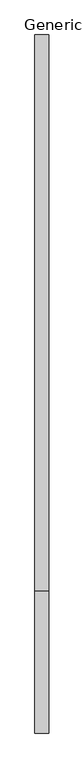
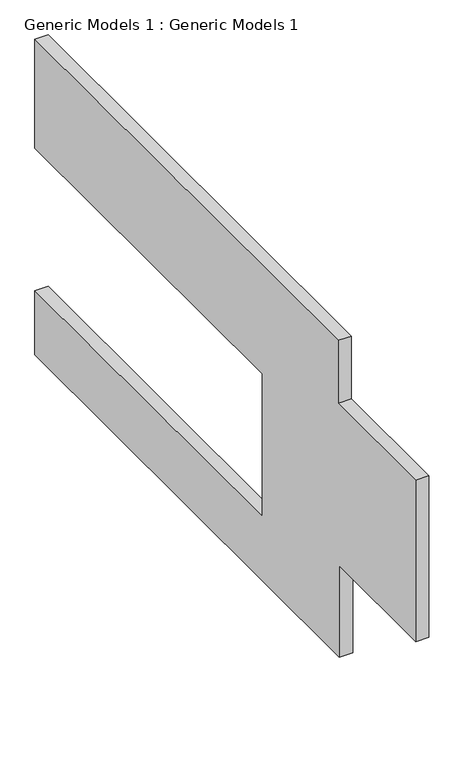
"""IFC4 building model written with IfcOpenShell, lengths in millimetres: proxy geometry, Generic Models 1 : Generic Models 1."""

from ifc_helpers import new_model, si_unit, frame, origin, place, context, project, spatial, polyline, outline, extrude, source, transform, mapped, element, save


def generic_models_1_generic_models_1_98a022ed(model_context):
    return source(origin(), model_context, "Body", "SweptSolid", [
        extrude(outline(polyline([(-3946.8023495, 0.0), (-3946.8023495, 2214.7139463), (-6979.1363705, 2214.7139463), (-6979.1363705, 6127.75), (-3899.3863708, 6127.75), (-3899.3863708, 7651.75), (8140.2136292, 7651.75), (8140.2136292, 5015.8429185), (-883.1363705, 5015.8429185), (-883.1363705, 1555.75), (8140.2136292, 1555.75), (8140.2136292, 0.0), (-3946.8023495, 0.0)])), frame((13902.5156363, 0.0, 0.0), z_axis=(1.0, 0.0, 0.0), x_axis=(0.0, 1.0, 0.0)), (0.0, 0.0, 1.0), 304.8),
    ])


if __name__ == "__main__":
    model = new_model("IFC4")
    model_context = context("Model", 3, world=origin())
    ifc_project = project(units=[si_unit("LENGTHUNIT", "METRE", prefix="MILLI")], contexts=[model_context])
    site = spatial("IfcSite", under=ifc_project)
    building = spatial("IfcBuilding", under=site)
    placement = place(None, origin())
    generic_models_1_generic_models_1_shape = generic_models_1_generic_models_1_98a022ed(model_context)
    element("IfcBuildingElementProxy", 1, Name="Generic Models 1 : Generic Models 1", ObjectType="Generic Models 1 : Generic Models 1", at=placement, inside=building, context=model_context, shape_type="MappedRepresentation", body=[
        mapped(generic_models_1_generic_models_1_shape, transform((0.0, 0.0, 0.0), x_axis=(1.0, 0.0, 0.0), y_axis=(0.0, 1.0, 0.0), z_axis=(0.0, 0.0, 1.0))),
    ])
    save(model, "model.ifc")
